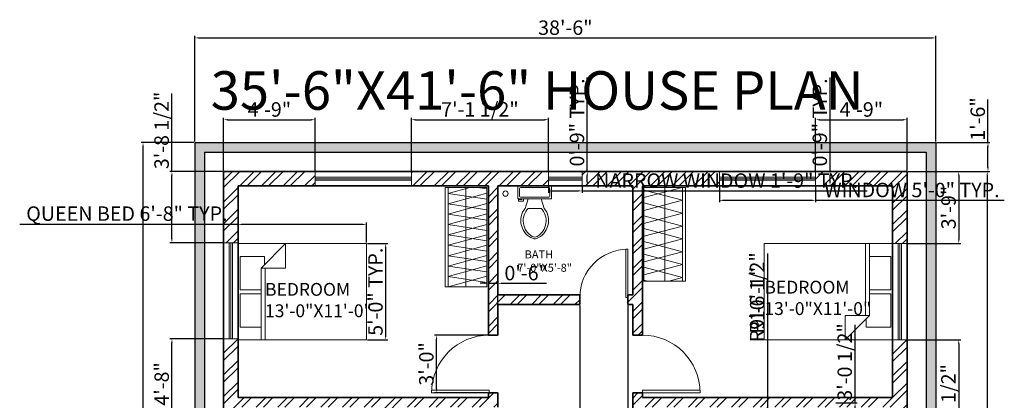
# Model space of a CAD drawing. Units: inches. Extents: x 418 to 1041, y 2094 to 2761.
# Tile 5 of 5: x 418 to 1032, y 2523 to 2761. Entities that reach past the tile are written whole.
import ezdxf

# ---------------------------------------------------------------- set-up
doc = ezdxf.new("R2010")
doc.units = ezdxf.units.IN
for name, color, linetype, lineweight in [('A-ANNO-DIMS', 2, 'Continuous', 18), ('A-ANNO-TEXT', 7, 'Continuous', 18), ('A-AREA-IDEN', 7, 'Continuous', 18), ('A-DOOR', 4, 'Continuous', 18), ('A-FLOR-CASE', 9, 'Continuous', 18), ('A-FLOR-CASE-PATT', 252, 'Continuous', 13), ('A-FLOR-FIXT', 9, 'Continuous', 18), ('A-FURN', 8, 'Continuous', 18), ('A-GLAZ', 244, 'Continuous', 18), ('A-WALL', 7, 'Continuous', 35), ('A-WALL-PATT', 252, 'Continuous', 13), ('L-WALL', 7, 'Continuous', 25), ('L-WALL-PATT', 252, 'Continuous', 13)]:
    doc.layers.add(name, color=color, linetype=linetype, lineweight=lineweight)
doc.styles.get("Standard").update_dxf_attribs({"font": 'arial.ttf'})
doc.dimstyles.new('ISO-25', dxfattribs={"dimtxt": 9, "dimasz": 2.5, "dimexe": 1.25, "dimexo": 0.625, "dimtad": 1, "dimlunit": 3, "dimtxsty": 'Standard', "dimcen": 2.5, "dimadec": 0, "dimazin": 0, "dimtfac": 1, "dimtmove": 0, "dimatfit": 3, "dimfxl": 1, "dimarcsym": 0})

# ---------------------------------------------------------------- blocks, each defined once
blk = doc.blocks.new('*U2')
for p, q in [((0, 0), (0, -6)), ((40, 0), (40, -6))]:
    blk.add_line(p, q)
blk.add_lwpolyline([(0, 0), (0, 40), (1.75, 40), (1.75, 0)], close=True)
blk.add_arc((0, 0), 40, 0, 90)
blk = doc.blocks.new('*U5')
for p, q in [((0, 0), (0, -6)), ((-40, 0), (-40, -6))]:
    blk.add_line(p, q)
blk.add_lwpolyline([(0, 0), (0, 40), (-1.75, 40), (-1.75, 0)], close=True)
blk.add_arc((0, 0), 40, 90, 180)
blk = doc.blocks.new('*U3')
for p, q in [((0, 0), (0, 6)), ((40, 0), (40, 6))]:
    blk.add_line(p, q)
blk.add_lwpolyline([(0, 0), (0, -40), (1.75, -40), (1.75, 0)], close=True)
blk.add_arc((0, 0), 40, 270, 0)
blk = doc.blocks.new('Bed - Queen')
for p, q in [((0, -80.00003), (0, 0)), ((0, 0), (59.99999, 0)), ((59.99999, 0), (59.99999, -80.00003)), ((7.99999, -1.2), (28.79998, -1.2)), ((7.99999, -14.4), (7.99999, -1.2)), ((28.79998, -1.2), (28.79998, -14.4)), ((31.19999, -1.2), (51.99999, -1.2)), ((31.19999, -14.4), (31.19999, -1.2)), ((51.99999, -1.2), (51.99999, -16.4)), ((0, -14.4), (44.8, -14.4)), ((44.8, -16.8), (0, -16.8)), ((59.99999, -29.6), (44.8, -14.4)), ((44.8, -14.4), (44.8, -29.6)), ((51.99999, -16.4), (46.79936, -16.4)), ((44.8, -29.6), (59.99999, -29.6)), ((59.99999, -80.00003), (0, -80.00003))]:
    blk.add_line(p, q)
blk = doc.blocks.new('*U10')
for p, q in [((9.5, -6), (9.5, -2)), ((-10, -8.5), (-8, -8.5)), ((-10, -9.5), (-10, -8.5)), ((-7, -9.5), (-10, -9.5)), ((-8, -8.5), (-8, -8)), ((-7, -8), (-7, -9.5)), ((-4, -8), (-6, -14)), ((4, -8), (6, -14)), ((4, -14), (-4, -14))]:
    blk.add_line(p, q)
blk.add_lwpolyline([(10.5, -8), (10.5, 0), (-10.5, 0), (-10.5, -8)], close=True)
for points in [[(-9.5, -2), (-9.5, -6)], [(8.5, -1), (-8.5, -1)], [(-8.5, -7), (8.5, -7)]]:
    blk.add_lwpolyline(points)
for centre, radius, start, end in [((-8.62, -1.88), 0.884, 81.8699, 188.1301), ((-8.62, -6.12), 0.884, 171.8699, 278.1301), ((8.62, -1.88), 0.884, 351.8699, 98.1301), ((8.62, -6.12), 0.884, 261.8699, 8.1301), ((3.52, -21.58), 12.17, 141.46911, 247.97143), ((4.2, -21.82), 11.33, 136.36773, 238.94682), ((-3.52, -21.58), 12.17, 292.02843, 38.53071), ((-4.2, -21.82), 11.33, 301.05301, 43.63209), ((0, -27.88), 4, 245.73182, 294.26817), ((0, -29), 4, 254.86053, 285.13947)]:
    blk.add_arc(centre, radius, start, end)
blk = doc.blocks.new('*D16')
at = {"layer": 'A-ANNO-DIMS', "color": 0, "lineweight": -2, "transparency": 16777216}
for p, q in [((972.18, 2666.03), (1022.79, 2666.03)), ((1021.54, 2663.53), (1021.54, 2170.53)), ((972.18, 2168.03), (1022.79, 2168.03))]:
    blk.add_line(p, q, dxfattribs=at)
at = {"layer": 'A-ANNO-DIMS', "color": 0, "transparency": 16777216}
for points in [[(1021.13, 2663.53), (1021.96, 2663.53), (1021.54, 2666.03)], [(1021.13, 2170.53), (1021.96, 2170.53), (1021.54, 2168.03)]]:
    blk.add_solid(points, dxfattribs=at)
at = {"layer": 'Defpoints', "color": 0, "transparency": 16777216}
for p in [(971.56, 2666.03), (971.56, 2168.03), (1021.54, 2168.03)]:
    blk.add_point(p, dxfattribs=at)
at = {"layer": 'A-ANNO-DIMS', "color": 0, "transparency": 16777216, "insert": (1016.32, 2417.03), "char_height": 9, "attachment_point": 5, "rotation": 90}
blk.add_mtext('41\'-6"', dxfattribs=at)
blk = doc.blocks.new('WIN-60IN')
for p, q in [((0, 5.5), (60, 5.5)), ((0, 4.5), (60, 4.5)), ((0, 3.5), (60, 3.5))]:
    blk.add_line(p, q)
blk.add_lwpolyline([(0, 9), (60, 9), (60, 0), (0, 0)], close=True)
blk = doc.blocks.new('WIN-21IN')
for p, q in [((0, 5.5), (21, 5.5)), ((0, 4.5), (21, 4.5)), ((0, 3.5), (21, 3.5))]:
    blk.add_line(p, q)
blk.add_lwpolyline([(0, 9), (21, 9), (21, 0), (0, 0)], close=True)
blk = doc.blocks.new('*D23')
at = {"layer": 'A-ANNO-DIMS', "color": 0, "lineweight": -2, "transparency": 16777216}
for p, q in [((854.56, 2656.4), (854.56, 2646.78)), ((914.56, 2656.4), (914.56, 2646.78)), ((857.06, 2648.03), (912.06, 2648.03)), ((914.56, 2648.03), (1032.2, 2648.03))]:
    blk.add_line(p, q, dxfattribs=at)
at = {"layer": 'A-ANNO-DIMS', "color": 0, "transparency": 16777216}
for points in [[(857.06, 2648.44), (857.06, 2647.61), (854.56, 2648.03)], [(912.06, 2648.44), (912.06, 2647.61), (914.56, 2648.03)]]:
    blk.add_solid(points, dxfattribs=at)
at = {"layer": 'Defpoints', "color": 0, "transparency": 16777216}
for p in [(854.56, 2657.03), (914.56, 2657.03), (914.56, 2648.03)]:
    blk.add_point(p, dxfattribs=at)
at = {"layer": 'A-ANNO-DIMS', "color": 0, "transparency": 16777216, "insert": (974.63, 2653.31), "char_height": 9, "attachment_point": 5}
blk.add_mtext('WINDOW 5\'-0" TYP.', dxfattribs=at)
blk = doc.blocks.new('*D24')
at = {"layer": 'A-ANNO-DIMS', "color": 0, "lineweight": -2, "transparency": 16777216}
for p, q in [((923.56, 2666.03), (923.56, 2724.63)), ((915.18, 2666.03), (924.81, 2666.03)), ((923.56, 2659.53), (923.56, 2663.53)), ((915.18, 2657.03), (924.81, 2657.03))]:
    blk.add_line(p, q, dxfattribs=at)
at = {"layer": 'A-ANNO-DIMS', "color": 0, "transparency": 16777216}
for points in [[(923.14, 2663.53), (923.97, 2663.53), (923.56, 2666.03)], [(923.14, 2659.53), (923.97, 2659.53), (923.56, 2657.03)]]:
    blk.add_solid(points, dxfattribs=at)
at = {"layer": 'Defpoints', "color": 0, "transparency": 16777216}
for p in [(914.56, 2666.03), (923.56, 2666.03), (914.56, 2657.03)]:
    blk.add_point(p, dxfattribs=at)
at = {"layer": 'A-ANNO-DIMS', "color": 0, "transparency": 16777216, "insert": (918.34, 2696.58), "char_height": 9, "attachment_point": 5, "rotation": 90}
blk.add_mtext('0\'-9" TYP.', dxfattribs=at)
blk = doc.blocks.new('*D25')
at = {"layer": 'A-ANNO-DIMS', "color": 0, "lineweight": -2, "transparency": 16777216}
for p, q in [((748.06, 2656.4), (748.06, 2652.63)), ((750.56, 2653.88), (766.56, 2653.88)), ((769.06, 2656.4), (769.06, 2652.63)), ((769.06, 2653.88), (946.66, 2653.88))]:
    blk.add_line(p, q, dxfattribs=at)
at = {"layer": 'A-ANNO-DIMS', "color": 0, "transparency": 16777216}
for points in [[(750.56, 2654.29), (750.56, 2653.46), (748.06, 2653.88)], [(766.56, 2654.29), (766.56, 2653.46), (769.06, 2653.88)]]:
    blk.add_solid(points, dxfattribs=at)
at = {"layer": 'Defpoints', "color": 0, "transparency": 16777216}
for p in [(748.06, 2657.03), (769.06, 2657.03), (769.06, 2653.88)]:
    blk.add_point(p, dxfattribs=at)
at = {"layer": 'A-ANNO-DIMS', "color": 0, "transparency": 16777216, "insert": (859.11, 2659.16), "char_height": 9, "attachment_point": 5}
blk.add_mtext('NARROW WINDOW 1\'-9" TYP.', dxfattribs=at)
blk = doc.blocks.new('*D26')
at = {"layer": 'A-ANNO-DIMS', "color": 0, "lineweight": -2, "transparency": 16777216}
for p, q in [((772.21, 2666.03), (772.21, 2724.63)), ((769.68, 2666.03), (773.46, 2666.03)), ((772.21, 2659.53), (772.21, 2663.53)), ((769.68, 2657.03), (773.46, 2657.03))]:
    blk.add_line(p, q, dxfattribs=at)
at = {"layer": 'A-ANNO-DIMS', "color": 0, "transparency": 16777216}
for points in [[(771.79, 2663.53), (772.62, 2663.53), (772.21, 2666.03)], [(771.79, 2659.53), (772.62, 2659.53), (772.21, 2657.03)]]:
    blk.add_solid(points, dxfattribs=at)
at = {"layer": 'Defpoints', "color": 0, "transparency": 16777216}
for p in [(769.06, 2666.03), (772.21, 2666.03), (769.06, 2657.03)]:
    blk.add_point(p, dxfattribs=at)
at = {"layer": 'A-ANNO-DIMS', "color": 0, "transparency": 16777216, "insert": (766.99, 2696.58), "char_height": 9, "attachment_point": 5, "rotation": 90}
blk.add_mtext('0\'-9" TYP.', dxfattribs=at)
blk = doc.blocks.new('*D27')
at = {"layer": 'A-ANNO-DIMS', "color": 0, "lineweight": -2, "transparency": 16777216}
for p, q in [((554.56, 2621.65), (554.56, 2634.28)), ((634.56, 2621.65), (634.56, 2634.28)), ((554.56, 2633.03), (418.42, 2633.03)), ((632.06, 2633.03), (557.06, 2633.03))]:
    blk.add_line(p, q, dxfattribs=at)
at = {"layer": 'A-ANNO-DIMS', "color": 0, "transparency": 16777216}
for points in [[(557.06, 2633.44), (557.06, 2632.61), (554.56, 2633.03)], [(632.06, 2633.44), (632.06, 2632.61), (634.56, 2633.03)]]:
    blk.add_solid(points, dxfattribs=at)
at = {"layer": 'Defpoints', "color": 0, "transparency": 16777216}
for p in [(554.56, 2633.03), (554.56, 2621.03), (634.56, 2621.03)]:
    blk.add_point(p, dxfattribs=at)
at = {"layer": 'A-ANNO-DIMS', "color": 0, "transparency": 16777216, "insert": (485.24, 2638.58), "char_height": 9, "attachment_point": 5}
blk.add_mtext('QUEEN BED 6\'-8" TYP.', dxfattribs=at)
blk = doc.blocks.new('*D28')
at = {"layer": 'A-ANNO-DIMS', "color": 0, "lineweight": -2, "transparency": 16777216}
for p, q in [((635.18, 2621.03), (647.81, 2621.03)), ((646.56, 2563.53), (646.56, 2618.53)), ((635.18, 2561.03), (647.81, 2561.03))]:
    blk.add_line(p, q, dxfattribs=at)
at = {"layer": 'A-ANNO-DIMS', "color": 0, "transparency": 16777216}
for points in [[(646.14, 2618.53), (646.97, 2618.53), (646.56, 2621.03)], [(646.14, 2563.53), (646.97, 2563.53), (646.56, 2561.03)]]:
    blk.add_solid(points, dxfattribs=at)
at = {"layer": 'Defpoints', "color": 0, "transparency": 16777216}
for p in [(634.56, 2621.03), (646.56, 2621.03), (634.56, 2561.03)]:
    blk.add_point(p, dxfattribs=at)
at = {"layer": 'A-ANNO-DIMS', "color": 0, "transparency": 16777216, "insert": (641.34, 2591.03), "char_height": 9, "attachment_point": 5, "rotation": 90}
blk.add_mtext('5\'-0" TYP.', dxfattribs=at)
blk = doc.blocks.new('*D38')
at = {"layer": 'A-ANNO-DIMS', "color": 0, "lineweight": -2, "transparency": 16777216}
for p, q in [((939.16, 2521.69), (939.16, 2570.33)), ((927.18, 2521.69), (940.41, 2521.69)), ((939.16, 2487.53), (939.16, 2519.19)), ((927.18, 2485.03), (940.41, 2485.03))]:
    blk.add_line(p, q, dxfattribs=at)
at = {"layer": 'A-ANNO-DIMS', "color": 0, "transparency": 16777216}
for points in [[(938.74, 2519.19), (939.57, 2519.19), (939.16, 2521.69)], [(938.74, 2487.53), (939.57, 2487.53), (939.16, 2485.03)]]:
    blk.add_solid(points, dxfattribs=at)
at = {"layer": 'Defpoints', "color": 0, "transparency": 16777216}
for p in [(926.56, 2521.69), (939.16, 2521.69), (926.56, 2485.03)]:
    blk.add_point(p, dxfattribs=at)
at = {"layer": 'A-ANNO-DIMS', "color": 0, "transparency": 16777216, "insert": (933.88, 2547.26), "char_height": 9, "attachment_point": 5, "rotation": 90}
blk.add_mtext('3\'-0 1/2"', dxfattribs=at)
blk = doc.blocks.new('*D41')
at = {"layer": 'A-ANNO-DIMS', "color": 0, "lineweight": -2, "transparency": 16777216}
for p, q in [((545.56, 2666.65), (545.56, 2699.53)), ((548.06, 2698.28), (600.06, 2698.28)), ((602.56, 2666.65), (602.56, 2699.53))]:
    blk.add_line(p, q, dxfattribs=at)
at = {"layer": 'A-ANNO-DIMS', "color": 0, "transparency": 16777216}
for points in [[(548.06, 2698.69), (548.06, 2697.86), (545.56, 2698.28)], [(600.06, 2698.69), (600.06, 2697.86), (602.56, 2698.28)]]:
    blk.add_solid(points, dxfattribs=at)
at = {"layer": 'Defpoints', "color": 0, "transparency": 16777216}
for p in [(602.56, 2698.28), (545.56, 2666.03), (602.56, 2666.03)]:
    blk.add_point(p, dxfattribs=at)
at = {"layer": 'A-ANNO-DIMS', "color": 0, "transparency": 16777216, "insert": (574.06, 2703.5), "char_height": 9, "attachment_point": 5}
blk.add_mtext('4\'-9"', dxfattribs=at)
blk = doc.blocks.new('*D42')
at = {"layer": 'A-ANNO-DIMS', "color": 0, "lineweight": -2, "transparency": 16777216}
for p, q in [((662.56, 2666.65), (662.56, 2699.53)), ((665.06, 2698.28), (745.56, 2698.28)), ((748.06, 2666.65), (748.06, 2699.53))]:
    blk.add_line(p, q, dxfattribs=at)
at = {"layer": 'A-ANNO-DIMS', "color": 0, "transparency": 16777216}
for points in [[(665.06, 2698.69), (665.06, 2697.86), (662.56, 2698.28)], [(745.56, 2698.69), (745.56, 2697.86), (748.06, 2698.28)]]:
    blk.add_solid(points, dxfattribs=at)
at = {"layer": 'Defpoints', "color": 0, "transparency": 16777216}
for p in [(748.06, 2698.28), (662.56, 2666.03), (748.06, 2666.03)]:
    blk.add_point(p, dxfattribs=at)
at = {"layer": 'A-ANNO-DIMS', "color": 0, "transparency": 16777216, "insert": (705.31, 2703.55), "char_height": 9, "attachment_point": 5}
blk.add_mtext('7\'-1 1/2"', dxfattribs=at)
blk = doc.blocks.new('*D43')
at = {"layer": 'A-ANNO-DIMS', "color": 0, "lineweight": -2, "transparency": 16777216}
for p, q in [((914.56, 2666.65), (914.56, 2699.53)), ((917.06, 2698.28), (969.06, 2698.28)), ((971.56, 2666.65), (971.56, 2699.53))]:
    blk.add_line(p, q, dxfattribs=at)
at = {"layer": 'A-ANNO-DIMS', "color": 0, "transparency": 16777216}
for points in [[(917.06, 2698.69), (917.06, 2697.86), (914.56, 2698.28)], [(969.06, 2698.69), (969.06, 2697.86), (971.56, 2698.28)]]:
    blk.add_solid(points, dxfattribs=at)
at = {"layer": 'Defpoints', "color": 0, "transparency": 16777216}
for p in [(971.56, 2698.28), (914.56, 2666.03), (971.56, 2666.03)]:
    blk.add_point(p, dxfattribs=at)
at = {"layer": 'A-ANNO-DIMS', "color": 0, "transparency": 16777216, "insert": (943.06, 2703.5), "char_height": 9, "attachment_point": 5}
blk.add_mtext('4\'-9"', dxfattribs=at)
blk = doc.blocks.new('*D44')
at = {"layer": 'A-ANNO-DIMS', "color": 0, "lineweight": -2, "transparency": 16777216}
for p, q in [((513.31, 2666.03), (513.31, 2714.66)), ((544.93, 2666.03), (512.06, 2666.03)), ((513.31, 2624.11), (513.31, 2663.53)), ((544.93, 2621.61), (512.06, 2621.61))]:
    blk.add_line(p, q, dxfattribs=at)
at = {"layer": 'A-ANNO-DIMS', "color": 0, "transparency": 16777216}
for points in [[(512.89, 2663.53), (513.72, 2663.53), (513.31, 2666.03)], [(512.89, 2624.11), (513.72, 2624.11), (513.31, 2621.61)]]:
    blk.add_solid(points, dxfattribs=at)
at = {"layer": 'Defpoints', "color": 0, "transparency": 16777216}
for p in [(513.31, 2666.03), (545.56, 2666.03), (545.56, 2621.61)]:
    blk.add_point(p, dxfattribs=at)
at = {"layer": 'A-ANNO-DIMS', "color": 0, "transparency": 16777216, "insert": (508.03, 2691.6), "char_height": 9, "attachment_point": 5, "rotation": 90}
blk.add_mtext('3\'-8 1/2"', dxfattribs=at)
blk = doc.blocks.new('*D45')
at = {"layer": 'A-ANNO-DIMS', "color": 0, "lineweight": -2, "transparency": 16777216}
for p, q in [((544.93, 2561.61), (512.06, 2561.61)), ((513.31, 2508.03), (513.31, 2559.11)), ((544.93, 2505.53), (512.06, 2505.53))]:
    blk.add_line(p, q, dxfattribs=at)
at = {"layer": 'A-ANNO-DIMS', "color": 0, "transparency": 16777216}
for points in [[(512.89, 2559.11), (513.72, 2559.11), (513.31, 2561.61)], [(512.89, 2508.03), (513.72, 2508.03), (513.31, 2505.53)]]:
    blk.add_solid(points, dxfattribs=at)
at = {"layer": 'Defpoints', "color": 0, "transparency": 16777216}
for p in [(513.31, 2561.61), (545.56, 2561.61), (545.56, 2505.53)]:
    blk.add_point(p, dxfattribs=at)
at = {"layer": 'A-ANNO-DIMS', "color": 0, "transparency": 16777216, "insert": (508.09, 2533.57), "char_height": 9, "attachment_point": 5, "rotation": 90}
blk.add_mtext('4\'-8"', dxfattribs=at)
blk = doc.blocks.new('*D47')
at = {"layer": 'A-ANNO-DIMS', "color": 0, "lineweight": -2, "transparency": 16777216}
for p, q in [((972.18, 2666.03), (1005.06, 2666.03)), ((1003.81, 2663.53), (1003.81, 2623.53)), ((972.18, 2621.03), (1005.06, 2621.03))]:
    blk.add_line(p, q, dxfattribs=at)
at = {"layer": 'A-ANNO-DIMS', "color": 0, "transparency": 16777216}
for points in [[(1003.39, 2663.53), (1004.22, 2663.53), (1003.81, 2666.03)], [(1003.39, 2623.53), (1004.22, 2623.53), (1003.81, 2621.03)]]:
    blk.add_solid(points, dxfattribs=at)
at = {"layer": 'Defpoints', "color": 0, "transparency": 16777216}
for p in [(971.56, 2666.03), (971.56, 2621.03), (1003.81, 2621.03)]:
    blk.add_point(p, dxfattribs=at)
at = {"layer": 'A-ANNO-DIMS', "color": 0, "transparency": 16777216, "insert": (998.58, 2643.53), "char_height": 9, "attachment_point": 5, "rotation": 90}
blk.add_mtext('3\'-9"', dxfattribs=at)
blk = doc.blocks.new('*D48')
at = {"layer": 'A-ANNO-DIMS', "color": 0, "lineweight": -2, "transparency": 16777216}
for p, q in [((972.18, 2561.03), (1005.06, 2561.03)), ((1003.81, 2558.53), (1003.81, 2485.03)), ((972.18, 2482.53), (1005.06, 2482.53))]:
    blk.add_line(p, q, dxfattribs=at)
at = {"layer": 'A-ANNO-DIMS', "color": 0, "transparency": 16777216}
for points in [[(1003.39, 2558.53), (1004.22, 2558.53), (1003.81, 2561.03)], [(1003.39, 2485.03), (1004.22, 2485.03), (1003.81, 2482.53)]]:
    blk.add_solid(points, dxfattribs=at)
at = {"layer": 'Defpoints', "color": 0, "transparency": 16777216}
for p in [(971.56, 2561.03), (971.56, 2482.53), (1003.81, 2482.53)]:
    blk.add_point(p, dxfattribs=at)
at = {"layer": 'A-ANNO-DIMS', "color": 0, "transparency": 16777216, "insert": (998.53, 2521.78), "char_height": 9, "attachment_point": 5, "rotation": 90}
blk.add_mtext('6\'-6 1/2"', dxfattribs=at)
blk = doc.blocks.new('*D58')
at = {"layer": 'A-ANNO-DIMS', "color": 0, "lineweight": -2, "transparency": 16777216}
for p, q in [((709.93, 2564.03), (677.06, 2564.03)), ((678.31, 2530.53), (678.31, 2561.53)), ((709.93, 2528.03), (677.06, 2528.03))]:
    blk.add_line(p, q, dxfattribs=at)
at = {"layer": 'A-ANNO-DIMS', "color": 0, "transparency": 16777216}
for points in [[(677.89, 2561.53), (678.72, 2561.53), (678.31, 2564.03)], [(677.89, 2530.53), (678.72, 2530.53), (678.31, 2528.03)]]:
    blk.add_solid(points, dxfattribs=at)
at = {"layer": 'Defpoints', "color": 0, "transparency": 16777216}
for p in [(678.31, 2564.03), (710.56, 2564.03), (710.56, 2528.03)]:
    blk.add_point(p, dxfattribs=at)
at = {"layer": 'A-ANNO-DIMS', "color": 0, "transparency": 16777216, "insert": (673.08, 2546.03), "char_height": 9, "attachment_point": 5, "rotation": 90}
blk.add_mtext('3\'-0"', dxfattribs=at)
blk = doc.blocks.new('*D59')
at = {"layer": 'A-ANNO-DIMS', "color": 0, "lineweight": -2, "transparency": 16777216}
for p, q in [((767.56, 2582.4), (767.56, 2100.53)), ((797.56, 2582.4), (797.56, 2100.53)), ((770.06, 2101.78), (795.06, 2101.78))]:
    blk.add_line(p, q, dxfattribs=at)
at = {"layer": 'A-ANNO-DIMS', "color": 0, "transparency": 16777216}
for points in [[(770.06, 2102.19), (770.06, 2101.36), (767.56, 2101.78)], [(795.06, 2102.19), (795.06, 2101.36), (797.56, 2101.78)]]:
    blk.add_solid(points, dxfattribs=at)
at = {"layer": 'Defpoints', "color": 0, "transparency": 16777216}
for p in [(767.56, 2583.03), (797.56, 2583.03), (797.56, 2101.78)]:
    blk.add_point(p, dxfattribs=at)
at = {"layer": 'A-ANNO-DIMS', "color": 0, "transparency": 16777216, "insert": (782.56, 2107), "char_height": 9, "attachment_point": 5}
blk.add_mtext('2\'-6"', dxfattribs=at)
blk = doc.blocks.new('*D60')
at = {"layer": 'A-ANNO-DIMS', "color": 0, "lineweight": -2, "transparency": 16777216}
for p, q in [((527.56, 2684.65), (527.56, 2750.53)), ((989.56, 2684.65), (989.56, 2750.53)), ((530.06, 2749.28), (987.06, 2749.28))]:
    blk.add_line(p, q, dxfattribs=at)
at = {"layer": 'A-ANNO-DIMS', "color": 0, "transparency": 16777216}
for points in [[(530.06, 2749.69), (530.06, 2748.86), (527.56, 2749.28)], [(987.06, 2749.69), (987.06, 2748.86), (989.56, 2749.28)]]:
    blk.add_solid(points, dxfattribs=at)
at = {"layer": 'Defpoints', "color": 0, "transparency": 16777216}
for p in [(989.56, 2749.28), (527.56, 2684.03), (989.56, 2684.03)]:
    blk.add_point(p, dxfattribs=at)
at = {"layer": 'A-ANNO-DIMS', "color": 0, "transparency": 16777216, "insert": (758.56, 2754.5), "char_height": 9, "attachment_point": 5}
blk.add_mtext('38\'-6"', dxfattribs=at)
blk = doc.blocks.new('*D61')
at = {"layer": 'A-ANNO-DIMS', "color": 0, "lineweight": -2, "transparency": 16777216}
for p, q in [((526.93, 2684.03), (494.06, 2684.03)), ((495.31, 2137.53), (495.31, 2681.53)), ((526.93, 2135.03), (494.06, 2135.03))]:
    blk.add_line(p, q, dxfattribs=at)
at = {"layer": 'A-ANNO-DIMS', "color": 0, "transparency": 16777216}
for points in [[(494.89, 2681.53), (495.72, 2681.53), (495.31, 2684.03)], [(494.89, 2137.53), (495.72, 2137.53), (495.31, 2135.03)]]:
    blk.add_solid(points, dxfattribs=at)
at = {"layer": 'Defpoints', "color": 0, "transparency": 16777216}
for p in [(495.31, 2684.03), (527.56, 2684.03), (527.56, 2135.03)]:
    blk.add_point(p, dxfattribs=at)
at = {"layer": 'A-ANNO-DIMS', "color": 0, "transparency": 16777216, "insert": (490.09, 2409.53), "char_height": 9, "attachment_point": 5, "rotation": 90}
blk.add_mtext('45\'-9"', dxfattribs=at)
blk = doc.blocks.new('*D65')
at = {"layer": 'A-ANNO-DIMS', "color": 0, "lineweight": -2, "transparency": 16777216}
for p, q in [((710.56, 2564.65), (710.56, 2597.53)), ((716.56, 2564.65), (716.56, 2597.53)), ((708.06, 2596.28), (705.56, 2596.28)), ((710.56, 2596.28), (716.56, 2596.28)), ((719.06, 2596.28), (746.73, 2596.28))]:
    blk.add_line(p, q, dxfattribs=at)
at = {"layer": 'A-ANNO-DIMS', "color": 0, "transparency": 16777216}
for points in [[(708.06, 2596.69), (708.06, 2595.86), (710.56, 2596.28)], [(719.06, 2596.69), (719.06, 2595.86), (716.56, 2596.28)]]:
    blk.add_solid(points, dxfattribs=at)
at = {"layer": 'Defpoints', "color": 0, "transparency": 16777216}
for p in [(716.56, 2596.28), (710.56, 2564.03), (716.56, 2564.03)]:
    blk.add_point(p, dxfattribs=at)
at = {"layer": 'A-ANNO-DIMS', "color": 0, "transparency": 16777216, "insert": (734.15, 2601.5), "char_height": 9, "attachment_point": 5}
blk.add_mtext('0\'-6"', dxfattribs=at)
blk = doc.blocks.new('*D67')
at = {"layer": 'A-ANNO-DIMS', "color": 0, "lineweight": -2, "transparency": 16777216}
for p, q in [((1022.01, 2684.03), (1022.01, 2710.85)), ((990.18, 2684.03), (1023.26, 2684.03)), ((1022.01, 2668.53), (1022.01, 2681.53)), ((972.18, 2666.03), (1023.26, 2666.03))]:
    blk.add_line(p, q, dxfattribs=at)
at = {"layer": 'A-ANNO-DIMS', "color": 0, "transparency": 16777216}
for points in [[(1021.6, 2681.53), (1022.43, 2681.53), (1022.01, 2684.03)], [(1021.6, 2668.53), (1022.43, 2668.53), (1022.01, 2666.03)]]:
    blk.add_solid(points, dxfattribs=at)
at = {"layer": 'Defpoints', "color": 0, "transparency": 16777216}
for p in [(989.56, 2684.03), (1022.01, 2684.03), (971.56, 2666.03)]:
    blk.add_point(p, dxfattribs=at)
at = {"layer": 'A-ANNO-DIMS', "color": 0, "transparency": 16777216, "insert": (1016.79, 2698.69), "char_height": 9, "attachment_point": 5, "rotation": 90}
blk.add_mtext('1\'-6"', dxfattribs=at)
blk = doc.blocks.new('*D70')
at = {"layer": 'A-ANNO-DIMS', "color": 0, "lineweight": -2, "transparency": 16777216}
for p, q in [((884.56, 2606.13), (884.56, 2515.53)), ((884.56, 2391.83), (884.56, 2513.03))]:
    blk.add_line(p, q, dxfattribs=at)
at = {"layer": 'A-ANNO-DIMS', "color": 0, "transparency": 16777216}
blk.add_solid([(884.14, 2515.53), (884.97, 2515.53), (884.56, 2513.03)], dxfattribs=at)
at = {"layer": 'Defpoints', "color": 0, "transparency": 16777216}
for p in [(884.56, 2513.03), (884.56, 2391.83)]:
    blk.add_point(p, dxfattribs=at)
at = {"layer": 'A-ANNO-DIMS', "color": 0, "transparency": 16777216, "insert": (879.34, 2585.74), "char_height": 9, "attachment_point": 5, "rotation": 90}
blk.add_mtext('R10\'-1"', dxfattribs=at)
blk = doc.blocks.new('*D71')
at = {"layer": 'A-ANNO-DIMS', "color": 0, "lineweight": -2, "transparency": 16777216}
for p, q in [((884.56, 2614.95), (884.56, 2521.53)), ((884.56, 2404.78), (884.56, 2519.03))]:
    blk.add_line(p, q, dxfattribs=at)
at = {"layer": 'A-ANNO-DIMS', "color": 0, "transparency": 16777216}
blk.add_solid([(884.14, 2521.53), (884.97, 2521.53), (884.56, 2519.03)], dxfattribs=at)
at = {"layer": 'Defpoints', "color": 0, "transparency": 16777216}
for p in [(884.56, 2519.03), (884.56, 2404.78)]:
    blk.add_point(p, dxfattribs=at)
at = {"layer": 'A-ANNO-DIMS', "color": 0, "transparency": 16777216, "insert": (879.28, 2587.58), "char_height": 9, "attachment_point": 5, "rotation": 90}
blk.add_mtext('R9\'-6 1/2"', dxfattribs=at)

msp = doc.modelspace()

# ---------------------------------------------------------------- hatches: boundary and pattern name
at = {"layer": 'A-FLOR-CASE-PATT'}
h = msp.add_hatch(dxfattribs=at)
h.set_pattern_fill('ANSI31', color=256, scale=1.96484, angle=-29.6745, style=0)
h.paths.add_polyline_path([(685.558, 2594.087), (709.558, 2594.087), (709.558, 2656.025), (685.558, 2656.025)])
h = msp.add_hatch(dxfattribs=at)
h.set_pattern_fill('ANSI31', color=256, scale=2.015259, angle=126.2562, style=0)
h.paths.add_polyline_path([(685.558, 2594.087), (709.558, 2594.087), (709.558, 2656.025), (685.558, 2656.025)])
h = msp.add_hatch(dxfattribs=at)
h.set_pattern_fill('ANSI31', color=256, scale=2.43957, angle=120.049, style=0)
h.paths.add_polyline_path([(807.558, 2597.699), (831.558, 2597.699), (831.558, 2656.025), (807.558, 2656.025)])
h = msp.add_hatch(dxfattribs=at)
h.set_pattern_fill('ANSI31', color=256, scale=2.44064, angle=-30.2076, style=0)
h.paths.add_polyline_path([(807.558, 2597.699), (831.558, 2597.699), (831.558, 2656.025), (807.558, 2656.025)])
at = {"layer": 'A-WALL-PATT'}
h = msp.add_hatch(dxfattribs=at)
h.set_pattern_fill('ANSI32', color=256)
h.paths.add_polyline_path([(671.558, 2308.025), (554.558, 2308.025), (554.558, 2366.352), (545.558, 2366.352), (545.558, 2168.025), (555.667, 2168.025), (555.667, 2177.025), (554.558, 2177.025), (554.558, 2302.025), (671.558, 2302.025)])
h.paths.add_polyline_path([(719.558, 2299.025), (722.558, 2299.025), (722.558, 2306.225), (722.558, 2308.025), (707.558, 2308.025), (707.558, 2302.025), (710.558, 2302.025), (710.558, 2177.025), (665.344, 2177.025), (665.344, 2168.025), (719.558, 2168.025)])
h.paths.add_polyline_path([(605.344, 2177.025), (576.667, 2177.025), (576.667, 2168.025), (605.344, 2168.025)], flags=17)
h.paths.add_polyline_path([(795.654, 2308.025), (770.558, 2308.025), (770.558, 2299.025), (795.654, 2299.025)])
h.paths.add_polyline_path([(971.558, 2333.525), (962.558, 2333.525), (962.558, 2308.025), (890.558, 2308.025), (890.558, 2311.025), (886.058, 2311.025), (884.558, 2311.025), (884.558, 2308.025), (855.654, 2308.025), (855.654, 2299.025), (962.558, 2299.025), (962.558, 2269.763), (971.558, 2269.763)])
h.paths.add_polyline_path([(971.558, 2209.763), (962.558, 2209.763), (962.558, 2168.025), (971.558, 2168.025)])
h.paths.add_polyline_path([(971.558, 2422.525), (962.558, 2422.525), (962.558, 2386.025), (845.558, 2386.025), (845.558, 2380.025), (884.558, 2380.025), (884.558, 2341.025), (890.558, 2341.025), (890.558, 2380.025), (962.558, 2380.025), (962.558, 2354.525), (971.558, 2354.525)])
h.paths.add_polyline_path([(716.558, 2471.025), (651.558, 2471.025), (651.558, 2474.025), (647.058, 2474.025), (645.558, 2474.025), (645.558, 2471.025), (554.558, 2471.025), (554.558, 2484.525), (545.558, 2484.525), (545.558, 2426.352), (554.558, 2426.352), (554.558, 2465.025), (716.558, 2465.025)])
h.paths.add_polyline_path([(554.558, 2561.611), (545.558, 2561.611), (545.558, 2505.525), (554.558, 2505.525), (554.558, 2519.025), (645.558, 2519.025), (645.558, 2504.025), (651.558, 2504.025), (651.558, 2519.025), (716.558, 2519.025), (716.558, 2528.025), (710.558, 2528.025), (710.558, 2525.025), (554.558, 2525.025)])
h.paths.add_polyline_path([(971.558, 2561.025), (962.558, 2561.025), (962.558, 2525.025), (806.558, 2525.025), (806.558, 2528.025), (800.558, 2528.025), (800.558, 2380.025), (809.558, 2380.025), (809.558, 2386.025), (806.558, 2386.025), (806.558, 2519.025), (962.558, 2519.025), (962.558, 2482.525), (971.558, 2482.525)])
h.paths.add_polyline_path([(854.558, 2666.025), (769.058, 2666.025), (769.058, 2657.025), (800.558, 2657.025), (800.558, 2589.025), (797.558, 2589.025), (797.558, 2583.025), (800.558, 2583.025), (800.558, 2564.025), (806.558, 2564.025), (806.558, 2657.025), (854.558, 2657.025)])
h.paths.add_polyline_path([(971.558, 2666.025), (914.558, 2666.025), (914.558, 2657.025), (962.558, 2657.025), (962.558, 2621.025), (971.558, 2621.025)])
h.paths.add_polyline_path([(748.058, 2666.025), (662.558, 2666.025), (662.558, 2657.025), (710.558, 2657.025), (710.558, 2564.025), (716.558, 2564.025), (716.558, 2583.025), (767.558, 2583.025), (767.558, 2589.025), (716.558, 2589.025), (716.558, 2657.025), (748.058, 2657.025)])
h.paths.add_polyline_path([(602.558, 2666.025), (545.558, 2666.025), (545.558, 2621.611), (554.558, 2621.611), (554.558, 2657.025), (602.558, 2657.025)])
at = {"layer": 'L-WALL-PATT'}
h = msp.add_hatch(color=256, dxfattribs=at)
h.dxf.hatch_style = 1
h.paths.add_polyline_path([(533.558, 2678.025), (983.558, 2678.025), (983.558, 2141.025), (902.558, 2141.025), (902.558, 2168.025), (893.558, 2168.025), (893.558, 2135.025), (926.558, 2135.025), (989.558, 2135.025), (989.558, 2684.025), (527.558, 2684.025), (527.558, 2135.025), (723.29, 2135.025), (732.29, 2135.025), (732.29, 2168.025), (723.29, 2168.025), (723.29, 2141.025), (533.558, 2141.025)])

# ---------------------------------------------------------------- linework, layer by layer
at = {"layer": 'A-FLOR-CASE'}
for p, q in [((683.558, 2656.025), (709.558, 2656.025)), ((683.558, 2656.025), (683.558, 2594.087)), ((685.558, 2656.025), (685.558, 2594.087)), ((696.558, 2594.087), (696.558, 2656.025)), ((709.558, 2656.025), (709.558, 2594.087)), ((807.558, 2656.025), (833.558, 2656.025)), ((807.558, 2656.025), (807.558, 2597.699)), ((820.558, 2597.699), (820.558, 2656.025)), ((831.558, 2656.025), (831.558, 2597.699)), ((833.558, 2656.025), (833.558, 2597.699)), ((833.558, 2597.699), (807.558, 2597.699)), ((683.558, 2594.087), (709.558, 2594.087))]:
    msp.add_line(p, q, dxfattribs=at)
at = {"layer": 'A-FLOR-FIXT'}
msp.add_circle((721.253, 2652.204), 1.656, dxfattribs=at)
at = {"layer": 'A-WALL'}
for p, q in [((545.558, 2666.025), (545.558, 2168.025)), ((545.558, 2666.025), (971.558, 2666.025)), ((971.558, 2666.025), (971.558, 2168.025)), ((554.558, 2657.025), (710.558, 2657.025)), ((554.558, 2657.025), (554.558, 2525.025)), ((710.558, 2657.025), (710.558, 2564.025)), ((716.558, 2657.025), (716.558, 2589.025)), ((716.558, 2657.025), (800.558, 2657.025)), ((800.558, 2657.025), (800.558, 2589.025)), ((806.558, 2657.025), (806.558, 2564.025)), ((806.558, 2657.025), (962.558, 2657.025)), ((962.558, 2657.025), (962.558, 2525.025)), ((716.558, 2589.025), (767.558, 2589.025)), ((767.558, 2583.025), (767.558, 2589.025)), ((797.558, 2583.025), (797.558, 2589.025)), ((797.558, 2589.025), (800.558, 2589.025)), ((716.558, 2583.025), (767.558, 2583.025)), ((716.558, 2583.025), (716.558, 2564.025)), ((797.558, 2583.025), (800.558, 2583.025)), ((800.558, 2583.025), (800.558, 2564.025)), ((710.558, 2564.025), (716.558, 2564.025)), ((806.558, 2564.025), (800.558, 2564.025)), ((554.558, 2525.025), (710.558, 2525.025)), ((710.558, 2528.025), (716.558, 2528.025)), ((710.558, 2528.025), (710.558, 2525.025)), ((716.558, 2528.025), (716.558, 2519.025)), ((806.558, 2528.025), (800.558, 2528.025)), ((800.558, 2528.025), (800.558, 2380.025)), ((806.558, 2528.025), (806.558, 2525.025)), ((806.558, 2525.025), (962.558, 2525.025))]:
    msp.add_line(p, q, dxfattribs=at)
at = {"layer": 'L-WALL'}
for p, q in [((527.558, 2684.025), (527.558, 2135.025)), ((527.558, 2684.025), (989.558, 2684.025)), ((989.558, 2684.025), (989.558, 2135.025)), ((533.558, 2678.025), (533.558, 2141.025)), ((533.558, 2678.025), (983.558, 2678.025)), ((983.558, 2678.025), (983.558, 2141.025))]:
    msp.add_line(p, q, dxfattribs=at)

# ---------------------------------------------------------------- block references
at = {"layer": 'A-DOOR', "xscale": 0.75, "yscale": 0.75, "zscale": 0.75}
msp.add_blockref('*U5', (797.558, 2587.525), dxfattribs=at)
at = {"layer": 'A-DOOR', "xscale": 0.9, "yscale": 0.9, "zscale": 0.9, "rotation": 89.99999999999982}
for name, p in [('*U2', (711.158, 2528.025)), ('*U3', (806.558, 2528.025))]:
    msp.add_blockref(name, p, dxfattribs=at)
at = {"layer": 'A-FLOR-FIXT'}
msp.add_blockref('*U10', (739.442, 2657.025), dxfattribs=at)
at = {"layer": 'A-FURN'}
for p, rotation in [((554.558, 2561.025), 90), ((962.558, 2621.025), 270)]:
    msp.add_blockref('Bed - Queen', p, dxfattribs=dict(at, rotation=rotation))
at = {"layer": 'A-GLAZ'}
for name, p in [('WIN-60IN', (602.558, 2657.025)), ('WIN-21IN', (748.058, 2657.025)), ('WIN-60IN', (854.558, 2657.025))]:
    msp.add_blockref(name, p, dxfattribs=at)
for p, rotation in [((545.558, 2621.611), 270.000000000001), ((962.558, 2621.025), 270.0000000000006)]:
    msp.add_blockref('WIN-60IN', p, dxfattribs=dict(at, rotation=rotation))

# ---------------------------------------------------------------- texts
at = {"layer": 'A-ANNO-TEXT', "insert": (537.497, 2728.5), "char_height": 24, "attachment_point": 1}
msp.add_mtext_dynamic_manual_height_columns('35\'-6"X41\'-6" HOUSE PLAN', width=424.16193, gutter_width=12.5, heights=[0], dxfattribs=at)
at = {"layer": 'A-AREA-IDEN', "attachment_point": 1}
for s, width, insert, char_height in [('   BATH\\P7\'-0"X5\'-8"', 32.17073, (728.636, 2616.813), 5), ('BEDROOM\\P13\'-0"X11\'-0"', 63.10181, (571.358, 2596.514), 8), ('BEDROOM\\P13\'-0"X11\'-0"', 63.10181, (882.656, 2597.875), 8)]:
    msp.add_mtext_dynamic_manual_height_columns(s, width=width, gutter_width=12.5, heights=[0], dxfattribs=dict(at, insert=insert, char_height=char_height))

# ---------------------------------------------------------------- dimensions: what is measured, and where the dimension line sits
at = {"layer": 'A-ANNO-DIMS'}
for base, p1, p2, picture, middle in [((989.558, 2749.275), (527.558, 2684.025), (989.558, 2684.025), '*D60', (758.558, 2754.499)), ((748.058, 2698.275), (662.558, 2666.025), (748.058, 2666.025), '*D42', (705.308, 2703.554)), ((602.558, 2698.275), (545.558, 2666.025), (602.558, 2666.025), '*D41', (574.058, 2703.496)), ((716.558, 2596.275), (710.558, 2564.025), (716.558, 2564.025), '*D65', (734.145, 2601.496)), ((797.558, 2101.775), (767.558, 2583.025), (797.558, 2583.025), '*D59', (782.558, 2106.996))]:
    dim = msp.add_linear_dim(base=base, p1=p1, p2=p2, dimstyle='ISO-25', override={"dimdec": 1, "dimlfac": 1, "dimrnd": 0, "dimzin": 1, "dimdsep": 46, "dimlunit": 4, "dimfrac": 2}, dxfattribs=at)
    dim.commit()
    dim.dimension.update_dxf_attribs({"geometry": picture, "text_midpoint": middle})
for base, p1, p2, angle, text, picture, middle in [((772.208, 2666.025), (769.058, 2657.025), (769.058, 2666.025), 90, '<> TYP.', '*D26', (766.988, 2696.58)), ((923.558, 2666.025), (914.558, 2657.025), (914.558, 2666.025), 90, '<> TYP.', '*D24', (918.338, 2696.58)), ((554.558, 2633.025), (634.558, 2621.025), (554.558, 2621.025), 180, 'QUEEN BED <> TYP.', '*D27', (485.237, 2638.58)), ((646.558, 2621.025), (634.558, 2561.025), (634.558, 2621.025), 90, '<> TYP.', '*D28', (641.338, 2591.025))]:
    dim = msp.add_linear_dim(base=base, p1=p1, p2=p2, angle=angle, text=text, dimstyle='ISO-25', override={"dimdec": 1, "dimlfac": 1, "dimrnd": 0, "dimzin": 1, "dimdsep": 46, "dimlunit": 4, "dimfrac": 2}, dxfattribs=at)
    dim.commit()
    dim.dimension.update_dxf_attribs({"geometry": picture, "text_midpoint": middle})
for base, p1, p2, angle, override, picture, middle in [((513.308, 2666.025), (545.558, 2621.611), (545.558, 2666.025), 90, {"dimdec": 1, "dimlfac": 1, "dimrnd": 0, "dimzin": 1, "dimdsep": 46, "dimlunit": 4, "dimfrac": 2}, '*D44', (508.026, 2691.595)), ((971.558, 2698.275), (914.558, 2666.025), (971.558, 2666.025), 0, {"dimdec": 1, "dimlfac": 1, "dimrnd": 0, "dimzin": 1, "dimdsep": 46, "dimlunit": 4, "dimfrac": 2}, '*D43', (943.058, 2703.496)), ((1022.015, 2684.025), (971.558, 2666.025), (989.558, 2684.025), 90, {"dimdec": 1, "dimlfac": 1, "dimrnd": 0, "dimzin": 1, "dimdsep": 46, "dimlunit": 4, "dimfrac": 2}, '*D67', (1016.795, 2698.689)), ((495.308, 2684.025), (527.558, 2135.025), (527.558, 2684.025), 90, {"dimdec": 1, "dimlfac": 1, "dimrnd": 0, "dimzin": 1, "dimdsep": 46, "dimlunit": 4, "dimfrac": 2}, '*D61', (490.088, 2409.525)), ((1021.545, 2168.025), (971.558, 2666.025), (971.558, 2168.025), 90, {"dimclrd": 0, "dimclre": 0, "dimclrt": 0}, '*D16', (1016.325, 2417.025)), ((1003.808, 2621.025), (971.558, 2666.025), (971.558, 2621.025), 270, {"dimdec": 1, "dimlfac": 1, "dimrnd": 0, "dimzin": 1, "dimdsep": 46, "dimlunit": 4, "dimfrac": 2}, '*D47', (998.585, 2643.525)), ((939.158, 2521.692), (926.558, 2485.025), (926.558, 2521.692), 90, {"dimdec": 1, "dimlfac": 1, "dimrnd": 0, "dimzin": 1, "dimdsep": 46, "dimlunit": 4, "dimfrac": 2}, '*D38', (933.876, 2547.262)), ((513.308, 2561.611), (545.558, 2505.525), (545.558, 2561.611), 90, {"dimdec": 1, "dimlfac": 1, "dimrnd": 0, "dimzin": 1, "dimdsep": 46, "dimlunit": 4, "dimfrac": 2}, '*D45', (508.088, 2533.568)), ((678.308, 2564.025), (710.558, 2528.025), (710.558, 2564.025), 90, {"dimdec": 1, "dimlfac": 1, "dimrnd": 0, "dimzin": 1, "dimdsep": 46, "dimlunit": 4, "dimfrac": 2}, '*D58', (673.085, 2546.025)), ((1003.808, 2482.525), (971.558, 2561.025), (971.558, 2482.525), 270, {"dimdec": 1, "dimlfac": 1, "dimrnd": 0, "dimzin": 1, "dimdsep": 46, "dimlunit": 4, "dimfrac": 2}, '*D48', (998.529, 2521.775))]:
    dim = msp.add_linear_dim(base=base, p1=p1, p2=p2, angle=angle, dimstyle='ISO-25', override=override, dxfattribs=at)
    dim.commit()
    dim.dimension.update_dxf_attribs({"geometry": picture, "text_midpoint": middle})
for base, p1, p2, text, picture, middle in [((769.058, 2653.875), (748.058, 2657.025), (769.058, 2657.025), 'NARROW WINDOW <> TYP.', '*D25', (859.107, 2659.157)), ((914.558, 2648.025), (854.558, 2657.025), (914.558, 2657.025), 'WINDOW <> TYP.', '*D23', (974.627, 2653.307))]:
    dim = msp.add_linear_dim(base=base, p1=p1, p2=p2, text=text, dimstyle='ISO-25', override={"dimdec": 1, "dimlfac": 1, "dimrnd": 0, "dimzin": 1, "dimdsep": 46, "dimlunit": 4, "dimfrac": 2}, dxfattribs=at)
    dim.commit()
    dim.dimension.update_dxf_attribs({"geometry": picture, "text_midpoint": middle})
for center, mpoint, picture, middle in [((884.557902, 2404.775352), (884.558, 2519.025352), '*D71', (884.558, 2587.575352)), ((884.558, 2391.829), (884.558, 2513.025), '*D70', (884.558, 2585.743))]:
    dim = msp.add_radius_dim(center=center, mpoint=mpoint, dimstyle='ISO-25', override={"dimdec": 1, "dimlfac": 1, "dimrnd": 0, "dimzin": 1, "dimdsep": 46, "dimlunit": 4, "dimfrac": 2}, dxfattribs=at)
    dim.commit()
    dim.dimension.update_dxf_attribs({"geometry": picture, "text_midpoint": middle, "dimtype": 164})

doc.saveas('drawing.dxf')
